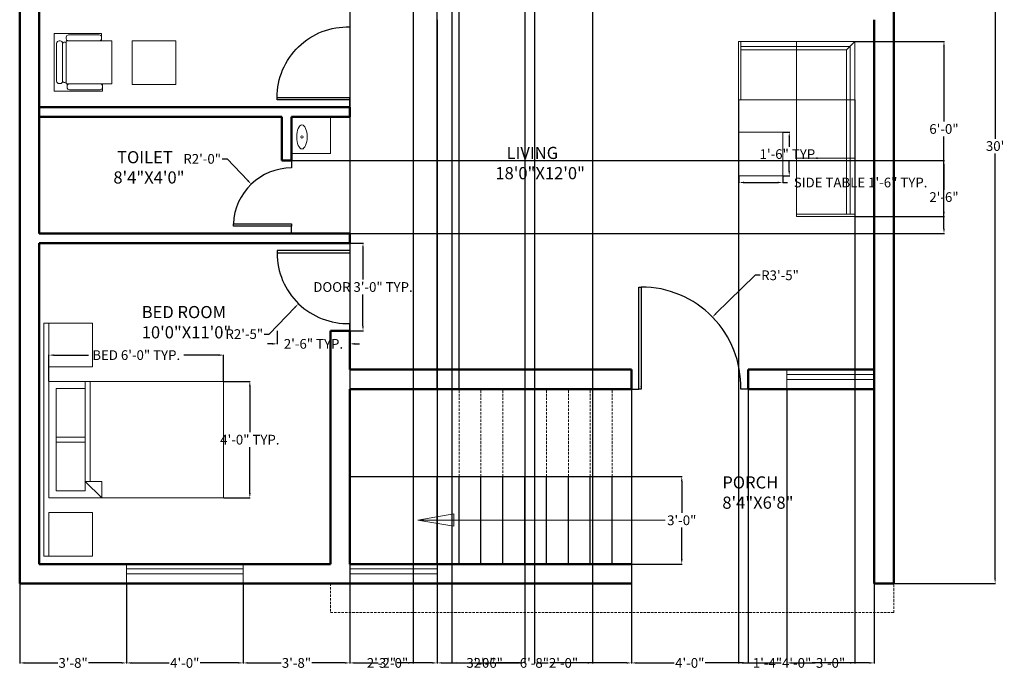
# Model space of a CAD drawing. Units: inches. Extents: x 284 to 690, y 63 to 494.
# Tile 1 of 2: x 284 to 690, y 63 to 331. Entities that reach past the tile are written whole.
import ezdxf

# ---------------------------------------------------------------- set-up
doc = ezdxf.new("R2010")
doc.units = ezdxf.units.IN
doc.header["$MEASUREMENT"] = 0
doc.linetypes.add('DASHEDX2', pattern=[1.5, 1, -0.5])
for name, color, linetype, lineweight in [('A-ANNO-DIMS', 2, 'Continuous', 18), ('A-ANNO-SYMB', 7, 'Continuous', 18), ('A-AREA-IDEN', 7, 'Continuous', 25), ('A-DOOR', 4, 'Continuous', 25), ('A-FLOR-FIXT', 9, 'Continuous', 18), ('A-FLOR-STRS', 7, 'Continuous', 25), ('A-FLOR-STRS-OVHD', 8, 'DASHEDX2', 18), ('A-FURN', 8, 'Continuous', 18), ('A-GLAZ', 3, 'Continuous', 18), ('A-ROOF-OVHD', 8, 'DASHEDX2', 18), ('A-WALL', 7, 'Continuous', 50)]:
    doc.layers.add(name, color=color, linetype=linetype, lineweight=lineweight)
doc.styles.get("Standard").update_dxf_attribs({"font": 'arial.ttf'})
doc.dimstyles.get("Standard").update_dxf_attribs({"dimtxt": 4, "dimasz": 2, "dimexe": 0.18, "dimexo": 0.0625, "dimgap": 1, "dimtad": 0, "dimtih": 1, "dimtoh": 1, "dimdec": 0, "dimzin": 0, "dimdsep": 46, "dimlunit": 3, "dimtxsty": 'Standard', "dimcen": 0.09, "dimadec": 0, "dimazin": 0, "dimtfac": 1, "dimtdec": 0, "dimtofl": 0, "dimtmove": 0, "dimatfit": 3, "dimfxl": 1, "dimtolj": 1, "dimtzin": 0, "dimarcsym": 0})

# ---------------------------------------------------------------- blocks, each defined once
blk = doc.blocks.new('*D2')
at = {"layer": 'A-ANNO-DIMS', "color": 0, "lineweight": -2, "transparency": 16777216}
for p, q in [((644.47, 458.55), (686.36, 458.55)), ((686.18, 456.55), (686.18, 281.59)), ((686.18, 100.55), (686.18, 275.51)), ((644.47, 98.55), (686.36, 98.55))]:
    blk.add_line(p, q, dxfattribs=at)
at = {"layer": 'A-ANNO-DIMS', "color": 0, "lineweight": -3, "transparency": 16777216}
for points in [[(685.85, 456.55), (686.51, 456.55), (686.18, 458.55)], [(685.85, 100.55), (686.51, 100.55), (686.18, 98.55)]]:
    blk.add_solid(points, dxfattribs=at)
at = {"layer": 'Defpoints', "color": 0, "lineweight": -3, "transparency": 16777216}
for p in [(644.41, 458.55), (644.41, 98.55), (686.18, 98.55)]:
    blk.add_point(p, dxfattribs=at)
at = {"layer": 'A-ANNO-DIMS', "color": 0, "transparency": 16777216, "insert": (686.18, 278.55), "char_height": 4, "attachment_point": 5}
blk.add_mtext("\\A1;30'", dxfattribs=at)
blk = doc.blocks.new('BED-48X72')
for p, q in [((0, 0), (0, 72)), ((0, 72), (48, 72)), ((23, 69), (23, 57)), ((25, 69), (25, 57)), ((45, 69), (45, 57)), ((48, 72), (48, 0)), ((0, 50.17), (6.83, 57)), ((45, 57), (3, 57)), ((6.83, 57), (6.83, 50.17)), ((45, 57), (48, 57)), ((48, 57), (48, 54)), ((48, 55), (6.83, 55)), ((0, 50.17), (6.83, 50.17)), ((48, 0), (0, 0))]:
    blk.add_line(p, q)
blk.add_lwpolyline([(3, 57), (3, 69), (45, 69), (45, 57)])
blk = doc.blocks.new('DOOR-SINGLE-30')
for p, q in [((30, 33), (0, 33)), ((0, 33), (0, 32)), ((30, 36), (30, 33)), ((30, 33), (30, 32)), ((0, 32), (30, 32)), ((30, 0), (30, 3))]:
    blk.add_line(p, q)
blk.add_arc((29.02, 32), 29.02, 180, 271.942)
blk = doc.blocks.new('TABLE-SIDE-18SQ')
blk.add_lwpolyline([(18, 18), (18, 0), (0, 0), (0, 18)], close=True)
blk = doc.blocks.new('*D7')
at = {"layer": 'A-ANNO-DIMS', "color": 0, "lineweight": -2, "transparency": 16777216}
for p, q in [((580.68, 266.19), (580.68, 263.37)), ((598.68, 266.19), (598.68, 263.37)), ((582.68, 263.55), (596.68, 263.55)), ((598.68, 263.55), (600.68, 263.55))]:
    blk.add_line(p, q, dxfattribs=at)
at = {"layer": 'A-ANNO-DIMS', "color": 0, "lineweight": -3, "transparency": 16777216}
for points in [[(582.68, 263.88), (582.68, 263.22), (580.68, 263.55)], [(596.68, 263.88), (596.68, 263.22), (598.68, 263.55)]]:
    blk.add_solid(points, dxfattribs=at)
at = {"layer": 'Defpoints', "color": 0, "lineweight": -3, "transparency": 16777216}
for p in [(580.68, 266.25), (598.68, 266.25), (598.68, 263.55)]:
    blk.add_point(p, dxfattribs=at)
at = {"layer": 'A-ANNO-DIMS', "color": 0, "transparency": 16777216, "insert": (630.78, 263.55), "char_height": 4, "attachment_point": 5}
blk.add_mtext('\\A1;SIDE TABLE 1\'-6" TYP.', dxfattribs=at)
blk = doc.blocks.new('*D8')
at = {"layer": 'A-ANNO-DIMS', "color": 0, "lineweight": -2, "transparency": 16777216}
for p, q in [((598.74, 284.25), (601.56, 284.25)), ((601.38, 282.25), (601.38, 278.29)), ((601.38, 268.25), (601.38, 272.21)), ((598.74, 266.25), (601.56, 266.25))]:
    blk.add_line(p, q, dxfattribs=at)
at = {"layer": 'A-ANNO-DIMS', "color": 0, "lineweight": -3, "transparency": 16777216}
for points in [[(601.04, 282.25), (601.71, 282.25), (601.38, 284.25)], [(601.04, 268.25), (601.71, 268.25), (601.38, 266.25)]]:
    blk.add_solid(points, dxfattribs=at)
at = {"layer": 'Defpoints', "color": 0, "lineweight": -3, "transparency": 16777216}
for p in [(598.68, 284.25), (601.38, 284.25), (598.68, 266.25)]:
    blk.add_point(p, dxfattribs=at)
at = {"layer": 'A-ANNO-DIMS', "color": 0, "transparency": 16777216, "insert": (601.38, 275.25), "char_height": 4, "attachment_point": 5}
blk.add_mtext('\\A1;1\'-6" TYP.', dxfattribs=at)
blk = doc.blocks.new('*D9')
at = {"layer": 'A-ANNO-DIMS', "color": 0, "lineweight": -2, "transparency": 16777216}
for p, q in [((296.41, 181.78), (296.41, 192.7)), ((298.41, 192.52), (312.78, 192.52)), ((366.41, 192.52), (352.03, 192.52)), ((368.41, 181.78), (368.41, 192.7))]:
    blk.add_line(p, q, dxfattribs=at)
at = {"layer": 'A-ANNO-DIMS', "color": 0, "lineweight": -3, "transparency": 16777216}
for points in [[(298.41, 192.85), (298.41, 192.19), (296.41, 192.52)], [(366.41, 192.85), (366.41, 192.19), (368.41, 192.52)]]:
    blk.add_solid(points, dxfattribs=at)
at = {"layer": 'Defpoints', "color": 0, "lineweight": -3, "transparency": 16777216}
for p in [(296.41, 192.52), (296.41, 181.72), (368.41, 181.72)]:
    blk.add_point(p, dxfattribs=at)
at = {"layer": 'A-ANNO-DIMS', "color": 0, "transparency": 16777216, "insert": (332.41, 192.52), "char_height": 4, "attachment_point": 5}
blk.add_mtext('\\A1;BED 6\'-0" TYP.', dxfattribs=at)
blk = doc.blocks.new('*D10')
at = {"layer": 'A-ANNO-DIMS', "color": 0, "lineweight": -2, "transparency": 16777216}
for p, q in [((368.47, 181.72), (379.39, 181.72)), ((379.21, 179.72), (379.21, 160.76)), ((379.21, 135.72), (379.21, 154.68)), ((368.47, 133.72), (379.39, 133.72))]:
    blk.add_line(p, q, dxfattribs=at)
at = {"layer": 'A-ANNO-DIMS', "color": 0, "lineweight": -3, "transparency": 16777216}
for points in [[(378.87, 179.72), (379.54, 179.72), (379.21, 181.72)], [(378.87, 135.72), (379.54, 135.72), (379.21, 133.72)]]:
    blk.add_solid(points, dxfattribs=at)
at = {"layer": 'Defpoints', "color": 0, "lineweight": -3, "transparency": 16777216}
for p in [(368.41, 181.72), (379.21, 181.72), (368.41, 133.72)]:
    blk.add_point(p, dxfattribs=at)
at = {"layer": 'A-ANNO-DIMS', "color": 0, "transparency": 16777216, "insert": (379.21, 157.72), "char_height": 4, "attachment_point": 5}
blk.add_mtext('\\A1;4\'-0" TYP.', dxfattribs=at)
blk = doc.blocks.new('*D11')
at = {"layer": 'A-ANNO-DIMS', "color": 0, "lineweight": -2, "transparency": 16777216}
for p, q in [((420.47, 238.55), (425.99, 238.55)), ((425.81, 236.55), (425.81, 223.62)), ((425.81, 204.55), (425.81, 217.48)), ((420.47, 202.55), (425.99, 202.55))]:
    blk.add_line(p, q, dxfattribs=at)
at = {"layer": 'A-ANNO-DIMS', "color": 0, "lineweight": -3, "transparency": 16777216}
for points in [[(425.47, 236.55), (426.14, 236.55), (425.81, 238.55)], [(425.47, 204.55), (426.14, 204.55), (425.81, 202.55)]]:
    blk.add_solid(points, dxfattribs=at)
at = {"layer": 'Defpoints', "color": 0, "lineweight": -3, "transparency": 16777216}
for p in [(420.41, 238.55), (425.81, 238.55), (420.41, 202.55)]:
    blk.add_point(p, dxfattribs=at)
at = {"layer": 'A-ANNO-DIMS', "color": 0, "transparency": 16777216, "insert": (425.81, 220.55), "char_height": 4, "attachment_point": 5}
blk.add_mtext('\\A1;DOOR 3\'-0" TYP.', dxfattribs=at)
blk = doc.blocks.new('*D12')
at = {"layer": 'A-ANNO-DIMS', "color": 0, "lineweight": -2, "transparency": 16777216}
for p, q in [((390.41, 202.49), (390.41, 196.97)), ((420.41, 202.49), (420.41, 196.97)), ((388.41, 197.15), (386.41, 197.15)), ((422.41, 197.15), (424.41, 197.15))]:
    blk.add_line(p, q, dxfattribs=at)
at = {"layer": 'A-ANNO-DIMS', "color": 0, "lineweight": -3, "transparency": 16777216}
for points in [[(388.41, 197.48), (388.41, 196.82), (390.41, 197.15)], [(422.41, 197.48), (422.41, 196.82), (420.41, 197.15)]]:
    blk.add_solid(points, dxfattribs=at)
at = {"layer": 'Defpoints', "color": 0, "lineweight": -3, "transparency": 16777216}
for p in [(390.41, 202.55), (420.41, 202.55), (420.41, 197.15)]:
    blk.add_point(p, dxfattribs=at)
at = {"layer": 'A-ANNO-DIMS', "color": 0, "transparency": 16777216, "insert": (405.41, 197.15), "char_height": 4, "attachment_point": 5}
blk.add_mtext('\\A1;2\'-6" TYP.', dxfattribs=at)
blk = doc.blocks.new('*D15')
at = {"layer": 'A-ANNO-DIMS', "color": 0, "lineweight": -2, "transparency": 16777216}
for p, q in [((284.41, 98.49), (284.41, 65.67)), ((328.41, 98.49), (328.41, 65.67)), ((286.41, 65.85), (300.09, 65.85)), ((326.41, 65.85), (312.72, 65.85))]:
    blk.add_line(p, q, dxfattribs=at)
at = {"layer": 'A-ANNO-DIMS', "color": 0, "lineweight": -3, "transparency": 16777216}
for points in [[(286.41, 66.18), (286.41, 65.52), (284.41, 65.85)], [(326.41, 66.18), (326.41, 65.52), (328.41, 65.85)]]:
    blk.add_solid(points, dxfattribs=at)
at = {"layer": 'Defpoints', "color": 0, "lineweight": -3, "transparency": 16777216}
for p in [(284.41, 98.55), (328.41, 98.55), (328.41, 65.85)]:
    blk.add_point(p, dxfattribs=at)
at = {"layer": 'A-ANNO-DIMS', "color": 0, "transparency": 16777216, "insert": (306.41, 65.85), "char_height": 4, "attachment_point": 5}
blk.add_mtext('\\A1;3\'-8"', dxfattribs=at)
blk = doc.blocks.new('*D16')
at = {"layer": 'A-ANNO-DIMS', "color": 0, "lineweight": -2, "transparency": 16777216}
for p, q in [((328.41, 98.49), (328.41, 65.67)), ((376.41, 98.49), (376.41, 65.67)), ((330.41, 65.85), (346.01, 65.85)), ((374.41, 65.85), (358.8, 65.85))]:
    blk.add_line(p, q, dxfattribs=at)
at = {"layer": 'A-ANNO-DIMS', "color": 0, "lineweight": -3, "transparency": 16777216}
for points in [[(330.41, 66.18), (330.41, 65.52), (328.41, 65.85)], [(374.41, 66.18), (374.41, 65.52), (376.41, 65.85)]]:
    blk.add_solid(points, dxfattribs=at)
at = {"layer": 'Defpoints', "color": 0, "lineweight": -3, "transparency": 16777216}
for p in [(328.41, 98.55), (376.41, 98.55), (376.41, 65.85)]:
    blk.add_point(p, dxfattribs=at)
at = {"layer": 'A-ANNO-DIMS', "color": 0, "transparency": 16777216, "insert": (352.41, 65.85), "char_height": 4, "attachment_point": 5}
blk.add_mtext('\\A1;4\'-0"', dxfattribs=at)
blk = doc.blocks.new('*D17')
at = {"layer": 'A-ANNO-DIMS', "color": 0, "lineweight": -2, "transparency": 16777216}
for p, q in [((376.41, 98.49), (376.41, 65.67)), ((420.41, 98.49), (420.41, 65.67)), ((378.41, 65.85), (392.09, 65.85)), ((418.41, 65.85), (404.72, 65.85))]:
    blk.add_line(p, q, dxfattribs=at)
at = {"layer": 'A-ANNO-DIMS', "color": 0, "lineweight": -3, "transparency": 16777216}
for points in [[(378.41, 66.18), (378.41, 65.52), (376.41, 65.85)], [(418.41, 66.18), (418.41, 65.52), (420.41, 65.85)]]:
    blk.add_solid(points, dxfattribs=at)
at = {"layer": 'Defpoints', "color": 0, "lineweight": -3, "transparency": 16777216}
for p in [(376.41, 98.55), (420.41, 98.55), (420.41, 65.85)]:
    blk.add_point(p, dxfattribs=at)
at = {"layer": 'A-ANNO-DIMS', "color": 0, "transparency": 16777216, "insert": (398.41, 65.85), "char_height": 4, "attachment_point": 5}
blk.add_mtext('\\A1;3\'-8"', dxfattribs=at)
blk = doc.blocks.new('*D18')
at = {"layer": 'A-ANNO-DIMS', "color": 0, "lineweight": -2, "transparency": 16777216}
for p, q in [((420.41, 98.49), (420.41, 65.67)), ((456.41, 98.49), (456.41, 65.67)), ((422.41, 65.85), (432.09, 65.85)), ((454.41, 65.85), (444.72, 65.85))]:
    blk.add_line(p, q, dxfattribs=at)
at = {"layer": 'A-ANNO-DIMS', "color": 0, "lineweight": -3, "transparency": 16777216}
for points in [[(422.41, 66.18), (422.41, 65.52), (420.41, 65.85)], [(454.41, 66.18), (454.41, 65.52), (456.41, 65.85)]]:
    blk.add_solid(points, dxfattribs=at)
at = {"layer": 'Defpoints', "color": 0, "lineweight": -3, "transparency": 16777216}
for p in [(420.41, 98.55), (456.41, 98.55), (456.41, 65.85)]:
    blk.add_point(p, dxfattribs=at)
at = {"layer": 'A-ANNO-DIMS', "color": 0, "transparency": 16777216, "insert": (438.41, 65.85), "char_height": 4, "attachment_point": 5}
blk.add_mtext('\\A1;3\'-0"', dxfattribs=at)
blk = doc.blocks.new('*D19')
at = {"layer": 'A-ANNO-DIMS', "color": 0, "lineweight": -2, "transparency": 16777216}
for p, q in [((456.41, 106.49), (456.41, 65.67)), ((536.41, 106.49), (536.41, 65.67)), ((458.41, 65.85), (490.08, 65.85)), ((534.41, 65.85), (502.73, 65.85))]:
    blk.add_line(p, q, dxfattribs=at)
at = {"layer": 'A-ANNO-DIMS', "color": 0, "lineweight": -3, "transparency": 16777216}
for points in [[(458.41, 66.18), (458.41, 65.52), (456.41, 65.85)], [(534.41, 66.18), (534.41, 65.52), (536.41, 65.85)]]:
    blk.add_solid(points, dxfattribs=at)
at = {"layer": 'Defpoints', "color": 0, "lineweight": -3, "transparency": 16777216}
for p in [(456.41, 106.55), (536.41, 106.55), (536.41, 65.85)]:
    blk.add_point(p, dxfattribs=at)
at = {"layer": 'A-ANNO-DIMS', "color": 0, "transparency": 16777216, "insert": (496.41, 65.85), "char_height": 4, "attachment_point": 5}
blk.add_mtext('\\A1;6\'-8"', dxfattribs=at)
blk = doc.blocks.new('*D20')
at = {"layer": 'A-ANNO-DIMS', "color": 0, "lineweight": -2, "transparency": 16777216}
for p, q in [((536.41, 178.49), (536.41, 65.67)), ((584.41, 178.49), (584.41, 65.67)), ((538.41, 65.85), (554.01, 65.85)), ((582.41, 65.85), (566.8, 65.85))]:
    blk.add_line(p, q, dxfattribs=at)
at = {"layer": 'A-ANNO-DIMS', "color": 0, "lineweight": -3, "transparency": 16777216}
for points in [[(538.41, 66.18), (538.41, 65.52), (536.41, 65.85)], [(582.41, 66.18), (582.41, 65.52), (584.41, 65.85)]]:
    blk.add_solid(points, dxfattribs=at)
at = {"layer": 'Defpoints', "color": 0, "lineweight": -3, "transparency": 16777216}
for p in [(536.41, 178.55), (584.41, 178.55), (584.41, 65.85)]:
    blk.add_point(p, dxfattribs=at)
at = {"layer": 'A-ANNO-DIMS', "color": 0, "transparency": 16777216, "insert": (560.41, 65.85), "char_height": 4, "attachment_point": 5}
blk.add_mtext('\\A1;4\'-0"', dxfattribs=at)
blk = doc.blocks.new('*D21')
at = {"layer": 'A-ANNO-DIMS', "color": 0, "lineweight": -2, "transparency": 16777216}
for p, q in [((584.41, 178.49), (584.41, 65.67)), ((600.41, 178.49), (600.41, 65.67)), ((582.41, 65.85), (580.41, 65.85)), ((602.41, 65.85), (604.41, 65.85))]:
    blk.add_line(p, q, dxfattribs=at)
at = {"layer": 'A-ANNO-DIMS', "color": 0, "lineweight": -3, "transparency": 16777216}
for points in [[(582.41, 66.18), (582.41, 65.52), (584.41, 65.85)], [(602.41, 66.18), (602.41, 65.52), (600.41, 65.85)]]:
    blk.add_solid(points, dxfattribs=at)
at = {"layer": 'Defpoints', "color": 0, "lineweight": -3, "transparency": 16777216}
for p in [(584.41, 178.55), (600.41, 178.55), (600.41, 65.85)]:
    blk.add_point(p, dxfattribs=at)
at = {"layer": 'A-ANNO-DIMS', "color": 0, "transparency": 16777216, "insert": (592.41, 65.85), "char_height": 4, "attachment_point": 5}
blk.add_mtext('\\A1;1\'-4"', dxfattribs=at)
blk = doc.blocks.new('*D22')
at = {"layer": 'A-ANNO-DIMS', "color": 0, "lineweight": -2, "transparency": 16777216}
for p, q in [((600.41, 178.49), (600.41, 65.67)), ((636.41, 178.49), (636.41, 65.67)), ((602.41, 65.85), (612.09, 65.85)), ((634.41, 65.85), (624.72, 65.85))]:
    blk.add_line(p, q, dxfattribs=at)
at = {"layer": 'A-ANNO-DIMS', "color": 0, "lineweight": -3, "transparency": 16777216}
for points in [[(602.41, 66.18), (602.41, 65.52), (600.41, 65.85)], [(634.41, 66.18), (634.41, 65.52), (636.41, 65.85)]]:
    blk.add_solid(points, dxfattribs=at)
at = {"layer": 'Defpoints', "color": 0, "lineweight": -3, "transparency": 16777216}
for p in [(600.41, 178.55), (636.41, 178.55), (636.41, 65.85)]:
    blk.add_point(p, dxfattribs=at)
at = {"layer": 'A-ANNO-DIMS', "color": 0, "transparency": 16777216, "insert": (618.41, 65.85), "char_height": 4, "attachment_point": 5}
blk.add_mtext('\\A1;3\'-0"', dxfattribs=at)
blk = doc.blocks.new('*D25')
at = {"layer": 'A-ANNO-DIMS', "color": 0, "lineweight": -2, "transparency": 16777216}
for p, q in [((456.41, 330.49), (456.41, 65.67)), ((492.41, 330.49), (492.41, 65.67)), ((458.41, 65.85), (468.09, 65.85)), ((490.41, 65.85), (480.72, 65.85))]:
    blk.add_line(p, q, dxfattribs=at)
at = {"layer": 'A-ANNO-DIMS', "color": 0, "lineweight": -3, "transparency": 16777216}
for points in [[(458.41, 66.18), (458.41, 65.52), (456.41, 65.85)], [(490.41, 66.18), (490.41, 65.52), (492.41, 65.85)]]:
    blk.add_solid(points, dxfattribs=at)
at = {"layer": 'Defpoints', "color": 0, "lineweight": -3, "transparency": 16777216}
for p in [(456.41, 330.55), (492.41, 330.55), (492.41, 65.85)]:
    blk.add_point(p, dxfattribs=at)
at = {"layer": 'A-ANNO-DIMS', "color": 0, "transparency": 16777216, "insert": (474.41, 65.85), "char_height": 4, "attachment_point": 5}
blk.add_mtext('\\A1;3\'-0"', dxfattribs=at)
blk = doc.blocks.new('*D26')
at = {"layer": 'A-ANNO-DIMS', "color": 0, "lineweight": -2, "transparency": 16777216}
for p, q in [((536.47, 142.55), (557.29, 142.55)), ((557.11, 140.55), (557.11, 127.59)), ((557.11, 108.55), (557.11, 121.51)), ((536.47, 106.55), (557.29, 106.55))]:
    blk.add_line(p, q, dxfattribs=at)
at = {"layer": 'A-ANNO-DIMS', "color": 0, "lineweight": -3, "transparency": 16777216}
for points in [[(556.77, 140.55), (557.44, 140.55), (557.11, 142.55)], [(556.77, 108.55), (557.44, 108.55), (557.11, 106.55)]]:
    blk.add_solid(points, dxfattribs=at)
at = {"layer": 'Defpoints', "color": 0, "lineweight": -3, "transparency": 16777216}
for p in [(536.41, 142.55), (536.41, 106.55), (557.11, 106.55)]:
    blk.add_point(p, dxfattribs=at)
at = {"layer": 'A-ANNO-DIMS', "color": 0, "transparency": 16777216, "insert": (557.11, 124.55), "char_height": 4, "attachment_point": 5}
blk.add_mtext('\\A1;3\'-0"', dxfattribs=at)
blk = doc.blocks.new('*D27')
at = {"layer": 'A-ANNO-DIMS', "color": 0, "lineweight": -2, "transparency": 16777216}
for p, q in [((456.41, 178.61), (456.41, 479.43)), ((458.41, 479.25), (463.41, 479.25)), ((465.41, 178.61), (465.41, 479.43)), ((465.41, 479.25), (467.41, 479.25))]:
    blk.add_line(p, q, dxfattribs=at)
at = {"layer": 'A-ANNO-DIMS', "color": 0, "lineweight": -3, "transparency": 16777216}
for points in [[(458.41, 479.58), (458.41, 478.92), (456.41, 479.25)], [(463.41, 479.58), (463.41, 478.92), (465.41, 479.25)]]:
    blk.add_solid(points, dxfattribs=at)
at = {"layer": 'Defpoints', "color": 0, "lineweight": -3, "transparency": 16777216}
for p in [(465.41, 479.25), (456.41, 178.55), (465.41, 178.55)]:
    blk.add_point(p, dxfattribs=at)
at = {"layer": 'A-ANNO-DIMS', "color": 0, "transparency": 16777216, "insert": (473.72, 479.25), "char_height": 4, "attachment_point": 5}
blk.add_mtext('\\A1;0\'-9"', dxfattribs=at)
blk = doc.blocks.new('*D28')
at = {"layer": 'A-ANNO-DIMS', "color": 0, "lineweight": -2, "transparency": 16777216}
for p, q in [((396.47, 272.55), (665.29, 272.55)), ((665.11, 270.55), (665.11, 260.59)), ((665.11, 244.55), (665.11, 254.51)), ((396.47, 242.55), (665.29, 242.55))]:
    blk.add_line(p, q, dxfattribs=at)
at = {"layer": 'A-ANNO-DIMS', "color": 0, "lineweight": -3, "transparency": 16777216}
for points in [[(664.77, 270.55), (665.44, 270.55), (665.11, 272.55)], [(664.77, 244.55), (665.44, 244.55), (665.11, 242.55)]]:
    blk.add_solid(points, dxfattribs=at)
at = {"layer": 'Defpoints', "color": 0, "lineweight": -3, "transparency": 16777216}
for p in [(396.41, 272.55), (665.11, 272.55), (396.41, 242.55)]:
    blk.add_point(p, dxfattribs=at)
at = {"layer": 'A-ANNO-DIMS', "color": 0, "transparency": 16777216, "insert": (665.11, 257.55), "char_height": 4, "attachment_point": 5}
blk.add_mtext('\\A1;2\'-6"', dxfattribs=at)
blk = doc.blocks.new('*D30')
at = {"layer": 'A-ANNO-DIMS', "color": 0, "lineweight": -2, "transparency": 16777216}
for p, q in [((496.41, 378.49), (496.41, 65.67)), ((520.41, 378.49), (520.41, 65.67)), ((498.41, 65.85), (502.06, 65.85)), ((518.41, 65.85), (514.76, 65.85))]:
    blk.add_line(p, q, dxfattribs=at)
at = {"layer": 'A-ANNO-DIMS', "color": 0, "lineweight": -3, "transparency": 16777216}
for points in [[(498.41, 66.18), (498.41, 65.52), (496.41, 65.85)], [(518.41, 66.18), (518.41, 65.52), (520.41, 65.85)]]:
    blk.add_solid(points, dxfattribs=at)
at = {"layer": 'Defpoints', "color": 0, "lineweight": -3, "transparency": 16777216}
for p in [(496.41, 378.55), (520.41, 378.55), (520.41, 65.85)]:
    blk.add_point(p, dxfattribs=at)
at = {"layer": 'A-ANNO-DIMS', "color": 0, "transparency": 16777216, "insert": (508.41, 65.85), "char_height": 4, "attachment_point": 5}
blk.add_mtext('\\A1;2\'-0"', dxfattribs=at)
blk = doc.blocks.new('*D32')
at = {"layer": 'A-ANNO-DIMS', "color": 0, "lineweight": -2, "transparency": 16777216}
for p, q in [((492.41, 390.49), (492.41, 65.67)), ((462.41, 386.49), (462.41, 65.67)), ((464.41, 65.85), (471.06, 65.85)), ((490.41, 65.85), (483.76, 65.85))]:
    blk.add_line(p, q, dxfattribs=at)
at = {"layer": 'A-ANNO-DIMS', "color": 0, "lineweight": -3, "transparency": 16777216}
for points in [[(464.41, 66.18), (464.41, 65.52), (462.41, 65.85)], [(490.41, 66.18), (490.41, 65.52), (492.41, 65.85)]]:
    blk.add_solid(points, dxfattribs=at)
at = {"layer": 'Defpoints', "color": 0, "lineweight": -3, "transparency": 16777216}
for p in [(492.41, 390.55), (462.41, 386.55), (492.41, 65.85)]:
    blk.add_point(p, dxfattribs=at)
at = {"layer": 'A-ANNO-DIMS', "color": 0, "transparency": 16777216, "insert": (477.41, 65.85), "char_height": 4, "attachment_point": 5}
blk.add_mtext('\\A1;2\'-6"', dxfattribs=at)
blk = doc.blocks.new('*D33')
at = {"layer": 'A-ANNO-DIMS', "color": 0, "lineweight": -2, "transparency": 16777216}
for p, q in [((420.41, 334.49), (420.41, 65.67)), ((446.41, 334.49), (446.41, 65.67)), ((422.41, 65.85), (427.06, 65.85)), ((444.41, 65.85), (439.76, 65.85))]:
    blk.add_line(p, q, dxfattribs=at)
at = {"layer": 'A-ANNO-DIMS', "color": 0, "lineweight": -3, "transparency": 16777216}
for points in [[(422.41, 66.18), (422.41, 65.52), (420.41, 65.85)], [(444.41, 66.18), (444.41, 65.52), (446.41, 65.85)]]:
    blk.add_solid(points, dxfattribs=at)
at = {"layer": 'Defpoints', "color": 0, "lineweight": -3, "transparency": 16777216}
for p in [(420.41, 334.55), (446.41, 334.55), (446.41, 65.85)]:
    blk.add_point(p, dxfattribs=at)
at = {"layer": 'A-ANNO-DIMS', "color": 0, "transparency": 16777216, "insert": (433.41, 65.85), "char_height": 4, "attachment_point": 5}
blk.add_mtext('\\A1;2\'-2"', dxfattribs=at)
blk = doc.blocks.new('*D34')
at = {"layer": 'A-ANNO-DIMS', "color": 0, "lineweight": -2, "transparency": 16777216}
for p, q in [((580.42, 297.53), (580.42, 65.67)), ((628.42, 297.53), (628.42, 65.67)), ((582.42, 65.85), (598.02, 65.85)), ((626.42, 65.85), (610.82, 65.85))]:
    blk.add_line(p, q, dxfattribs=at)
at = {"layer": 'A-ANNO-DIMS', "color": 0, "lineweight": -3, "transparency": 16777216}
for points in [[(582.42, 66.18), (582.42, 65.52), (580.42, 65.85)], [(626.42, 66.18), (626.42, 65.52), (628.42, 65.85)]]:
    blk.add_solid(points, dxfattribs=at)
at = {"layer": 'Defpoints', "color": 0, "lineweight": -3, "transparency": 16777216}
for p in [(580.42, 297.59), (628.42, 297.59), (628.42, 65.85)]:
    blk.add_point(p, dxfattribs=at)
at = {"layer": 'A-ANNO-DIMS', "color": 0, "transparency": 16777216, "insert": (604.42, 65.85), "char_height": 4, "attachment_point": 5}
blk.add_mtext('\\A1;4\'-0"', dxfattribs=at)
blk = doc.blocks.new('*D35')
at = {"layer": 'A-ANNO-DIMS', "color": 0, "lineweight": -2, "transparency": 16777216}
for p, q in [((628.48, 321.59), (665.29, 321.59)), ((665.11, 319.59), (665.11, 288.63)), ((665.11, 251.59), (665.11, 282.55)), ((628.48, 249.59), (665.29, 249.59))]:
    blk.add_line(p, q, dxfattribs=at)
at = {"layer": 'A-ANNO-DIMS', "color": 0, "lineweight": -3, "transparency": 16777216}
for points in [[(664.77, 319.59), (665.44, 319.59), (665.11, 321.59)], [(664.77, 251.59), (665.44, 251.59), (665.11, 249.59)]]:
    blk.add_solid(points, dxfattribs=at)
at = {"layer": 'Defpoints', "color": 0, "lineweight": -3, "transparency": 16777216}
for p in [(628.42, 321.59), (628.42, 249.59), (665.11, 249.59)]:
    blk.add_point(p, dxfattribs=at)
at = {"layer": 'A-ANNO-DIMS', "color": 0, "transparency": 16777216, "insert": (665.11, 285.59), "char_height": 4, "attachment_point": 5}
blk.add_mtext('\\A1;6\'-0"', dxfattribs=at)
blk = doc.blocks.new('*D36')
at = {"layer": 'A-ANNO-DIMS', "color": 0, "lineweight": -2, "transparency": 16777216}
for p, q in [((587.36, 225.37), (571.18, 209.58)), ((589.36, 225.37), (587.36, 225.37)), ((540.32, 179.54), (540.5, 179.54)), ((540.41, 179.45), (540.41, 179.63))]:
    blk.add_line(p, q, dxfattribs=at)
at = {"layer": 'A-ANNO-DIMS', "color": 0, "lineweight": -3, "transparency": 16777216}
blk.add_solid([(570.95, 209.82), (571.42, 209.34), (569.75, 208.19)], dxfattribs=at)
at = {"layer": 'Defpoints', "color": 0, "lineweight": -3, "transparency": 16777216}
for p in [(569.75, 208.19), (540.41, 179.54)]:
    blk.add_point(p, dxfattribs=at)
at = {"layer": 'A-ANNO-DIMS', "color": 0, "transparency": 16777216, "insert": (597.59, 225.37), "char_height": 4, "attachment_point": 5}
blk.add_mtext('\\A1;R3\'-5"', dxfattribs=at)
blk = doc.blocks.new('*D37')
at = {"layer": 'A-ANNO-DIMS', "color": 0, "lineweight": -2, "transparency": 16777216}
for p, q in [((419.33, 234.55), (419.51, 234.55)), ((419.42, 234.46), (419.42, 234.64)), ((387.15, 201.17), (397.86, 212.25)), ((385.15, 201.17), (387.15, 201.17))]:
    blk.add_line(p, q, dxfattribs=at)
at = {"layer": 'A-ANNO-DIMS', "color": 0, "lineweight": -3, "transparency": 16777216}
blk.add_solid([(397.63, 212.48), (398.1, 212.02), (399.26, 213.69)], dxfattribs=at)
at = {"layer": 'Defpoints', "color": 0, "lineweight": -3, "transparency": 16777216}
for p in [(419.42, 234.55), (399.26, 213.69)]:
    blk.add_point(p, dxfattribs=at)
at = {"layer": 'A-ANNO-DIMS', "color": 0, "transparency": 16777216, "insert": (376.92, 201.17), "char_height": 4, "attachment_point": 5}
blk.add_mtext('\\A1;R2\'-5"', dxfattribs=at)
blk = doc.blocks.new('*D38')
at = {"layer": 'A-ANNO-DIMS', "color": 0, "lineweight": -2, "transparency": 16777216}
for p, q in [((367.81, 273.28), (369.81, 273.28)), ((369.81, 273.28), (378.4, 264.32)), ((396.32, 245.53), (396.5, 245.53)), ((396.41, 245.44), (396.41, 245.62))]:
    blk.add_line(p, q, dxfattribs=at)
at = {"layer": 'A-ANNO-DIMS', "color": 0, "lineweight": -3, "transparency": 16777216}
blk.add_solid([(378.64, 264.55), (378.16, 264.08), (379.78, 262.87)], dxfattribs=at)
at = {"layer": 'Defpoints', "color": 0, "lineweight": -3, "transparency": 16777216}
for p in [(379.78, 262.87), (396.41, 245.53)]:
    blk.add_point(p, dxfattribs=at)
at = {"layer": 'A-ANNO-DIMS', "color": 0, "transparency": 16777216, "insert": (359.58, 273.28), "char_height": 4, "attachment_point": 5}
blk.add_mtext('\\A1;R2\'-0"', dxfattribs=at)

msp = doc.modelspace()

# ---------------------------------------------------------------- linework, layer by layer
at = {"layer": 'A-ANNO-SYMB'}
for p, q in [((448.41, 124.55), (463.18, 127.17)), ((463.18, 127.17), (463.2, 122.06)), ((456.41, 124.55), (448.41, 124.55)), ((448.41, 124.55), (463.2, 122.06)), ((456.41, 124.55), (550.22, 124.55))]:
    msp.add_line(p, q, dxfattribs=at)
at = {"layer": 'A-DOOR'}
for p, q in [((396.41, 272.55), (396.41, 269.55)), ((372.41, 245.55), (372.41, 246.55)), ((372.41, 246.55), (396.41, 246.55)), ((396.41, 245.55), (372.41, 245.55)), ((396.41, 246.55), (396.41, 245.55)), ((396.41, 242.55), (396.41, 245.55)), ((539.41, 178.55), (539.41, 220.55)), ((539.41, 220.55), (540.41, 220.55)), ((540.41, 220.55), (540.41, 178.55)), ((536.41, 178.55), (539.41, 178.55)), ((540.41, 178.55), (539.41, 178.55)), ((584.41, 178.55), (581.41, 178.55))]:
    msp.add_line(p, q, dxfattribs=at)
for centre, radius, start, end in [((396.41, 245.53), 24.02, 90, 177.5622), ((540.41, 179.54), 41.01, 358.6194, 90)]:
    msp.add_arc(centre, radius, start, end, dxfattribs=at)
at = {"layer": 'A-FLOR-FIXT'}
for p, q in [((412.41, 275.55), (412.41, 290.55)), ((396.41, 275.55), (412.41, 275.55))]:
    msp.add_line(p, q, dxfattribs=at)
msp.add_circle((400.67, 282.31), 0.5, dxfattribs=at)
msp.add_ellipse((400.67, 282.31), major_axis=(0, 4.94), ratio=0.435239, dxfattribs=at)
at = {"layer": 'A-FLOR-STRS'}
for p, q in [((420.41, 142.55), (536.41, 142.55)), ((456.41, 106.55), (456.41, 142.55)), ((465.41, 106.55), (465.41, 142.55)), ((474.41, 106.55), (474.41, 142.55)), ((483.41, 106.55), (483.41, 142.55)), ((492.41, 106.55), (492.41, 142.55)), ((501.41, 106.55), (501.41, 142.55)), ((510.41, 106.55), (510.41, 142.55)), ((510.41, 106.55), (510.41, 142.55)), ((510.41, 106.55), (510.41, 142.55)), ((519.41, 106.55), (519.41, 142.55)), ((528.41, 106.55), (528.41, 142.55)), ((536.41, 142.55), (536.41, 98.55)), ((420.41, 106.55), (456.41, 106.55))]:
    msp.add_line(p, q, dxfattribs=at)
at = {"layer": 'A-FLOR-STRS-OVHD'}
for p, q in [((456.41, 142.55), (456.41, 178.55)), ((465.41, 142.55), (465.41, 178.55)), ((474.41, 142.55), (474.41, 178.55)), ((483.41, 142.55), (483.41, 178.55)), ((492.41, 142.55), (492.41, 178.55)), ((501.41, 142.55), (501.41, 178.55)), ((510.41, 142.55), (510.41, 178.55)), ((519.41, 142.55), (519.41, 178.55)), ((528.41, 142.55), (528.41, 178.55)), ((536.41, 142.55), (536.41, 178.55))]:
    msp.add_line(p, q, dxfattribs=at)
at = {"layer": 'A-FURN'}
for p, q in [((299.63, 324.86), (298.63, 324.86)), ((298.63, 324.86), (298.63, 304.18)), ((318.14, 324.86), (299.63, 324.86)), ((318.14, 321.86), (318.14, 324.86)), ((299.63, 305.23), (299.63, 320.81)), ((300.63, 321.81), (301.1, 321.81)), ((302.1, 320.81), (302.1, 305.23)), ((302.1, 305.23), (302.1, 320.81)), ((302.6, 321.31), (303.06, 321.31)), ((303.56, 323.33), (303.56, 322.86)), ((303.56, 321.86), (310.85, 321.86)), ((303.56, 304.18), (303.56, 321.86)), ((303.56, 320.81), (303.56, 305.23)), ((310.85, 324.33), (304.56, 324.33)), ((304.56, 321.86), (310.85, 321.86)), ((317.14, 324.33), (310.85, 324.33)), ((310.85, 321.86), (317.14, 321.86)), ((310.85, 321.86), (322.39, 321.86)), ((318.14, 322.86), (318.14, 323.33)), ((322.39, 321.86), (322.39, 304.18)), ((604.42, 321.59), (580.42, 321.59)), ((580.42, 321.59), (580.42, 297.59)), ((581.42, 321.59), (581.42, 297.59)), ((628.42, 321.59), (604.42, 321.59)), ((604.42, 321.59), (604.42, 249.59)), ((624.92, 318.09), (628.42, 321.59)), ((628.42, 249.59), (628.42, 321.59)), ((604.42, 319.59), (581.42, 319.59)), ((604.42, 318.09), (581.42, 318.09)), ((626.42, 319.59), (604.42, 319.59)), ((624.92, 318.09), (604.42, 318.09)), ((624.92, 250.59), (624.92, 318.09)), ((626.42, 250.59), (626.42, 319.59)), ((298.63, 304.18), (298.63, 301.18)), ((301.1, 304.23), (300.63, 304.23)), ((303.06, 304.73), (302.6, 304.73)), ((310.85, 304.18), (303.56, 304.18)), ((310.85, 304.18), (304.93, 304.18)), ((322.39, 304.18), (310.85, 304.18)), ((317.5, 304.18), (310.85, 304.18)), ((310.85, 304.18), (310.85, 304.18)), ((310.85, 304.18), (310.85, 304.18)), ((318.5, 301.18), (318.5, 304.18)), ((298.63, 301.18), (318.5, 301.18)), ((303.93, 303.18), (303.93, 302.72)), ((304.93, 301.72), (310.85, 301.72)), ((310.85, 301.72), (317.5, 301.72)), ((318.5, 302.72), (318.5, 303.18)), ((580.42, 297.59), (604.42, 297.59)), ((604.42, 297.59), (628.42, 297.59)), ((604.42, 273.59), (628.42, 273.59)), ((604.42, 250.59), (628.42, 250.59)), ((604.42, 249.59), (628.42, 249.59)), ((294.41, 109.72), (294.41, 205.72)), ((296.41, 205.72), (294.41, 205.72)), ((296.41, 109.72), (294.41, 109.72))]:
    msp.add_line(p, q, dxfattribs=at)
for centre, radius, start, end in [((300.63, 320.81), 1, 90, 180), ((301.1, 320.81), 1, 0, 90), ((302.6, 320.81), 0.5, 90, 180), ((303.06, 320.81), 0.5, 0, 90), ((304.56, 323.33), 1, 90, 180), ((304.56, 322.86), 1, 180, 270), ((317.14, 323.33), 1, 0, 90), ((317.14, 322.86), 1, 270, 0), ((300.63, 305.23), 1, 180, 270), ((301.1, 305.23), 1, 270, 0), ((302.6, 305.23), 0.5, 180, 270), ((303.06, 305.23), 0.5, 270, 0), ((304.93, 303.18), 1, 90, 180), ((317.5, 303.18), 1, 0, 90), ((304.93, 302.72), 1, 180, 270), ((317.5, 302.72), 1, 270, 0)]:
    msp.add_arc(centre, radius, start, end, dxfattribs=at)
at = {"layer": 'A-GLAZ'}
for p, q in [((600.41, 178.55), (600.41, 186.55)), ((600.41, 184.55), (636.41, 184.55)), ((600.41, 182.55), (636.41, 182.55)), ((328.41, 106.55), (328.41, 98.55)), ((376.41, 106.55), (376.41, 98.55)), ((420.41, 106.55), (420.41, 98.55)), ((456.41, 106.55), (456.41, 98.55)), ((328.41, 104.55), (376.41, 104.55)), ((328.41, 102.55), (376.41, 102.55)), ((420.41, 104.55), (456.41, 104.55)), ((420.41, 102.55), (456.41, 102.55))]:
    msp.add_line(p, q, dxfattribs=at)
at = {"layer": 'A-ROOF-OVHD'}
for p, q in [((412.41, 98.55), (412.41, 86.55)), ((644.41, 86.55), (644.41, 98.55)), ((412.41, 86.55), (644.41, 86.55))]:
    msp.add_line(p, q, dxfattribs=at)
at = {"layer": 'A-WALL'}
for p, q in [((284.41, 98.55), (284.41, 458.55)), ((644.41, 458.55), (644.41, 98.55)), ((292.41, 242.55), (292.41, 450.55)), ((636.41, 98.55), (636.41, 330.55)), ((420.41, 294.55), (292.41, 294.55)), ((420.41, 290.55), (420.41, 294.55)), ((392.41, 290.55), (292.41, 290.55)), ((392.41, 290.55), (392.41, 272.55)), ((420.41, 290.55), (396.41, 290.55)), ((396.41, 290.55), (396.41, 272.55)), ((392.41, 272.55), (396.41, 272.55)), ((420.41, 242.55), (292.41, 242.55)), ((420.41, 242.55), (420.41, 238.55)), ((292.41, 106.55), (292.41, 238.55)), ((420.41, 238.55), (292.41, 238.55)), ((412.41, 106.55), (412.41, 202.55)), ((412.41, 202.55), (420.41, 202.55)), ((420.41, 186.55), (420.41, 202.55)), ((536.41, 186.55), (420.41, 186.55)), ((536.41, 178.55), (536.41, 186.55)), ((636.41, 186.55), (584.41, 186.55)), ((584.41, 178.55), (584.41, 186.55)), ((420.41, 106.55), (420.41, 178.55)), ((536.41, 178.55), (420.41, 178.55)), ((636.41, 178.55), (584.41, 178.55)), ((412.41, 106.55), (292.41, 106.55)), ((536.41, 106.55), (420.41, 106.55)), ((536.41, 98.55), (284.41, 98.55)), ((644.41, 98.55), (636.41, 98.55))]:
    msp.add_line(p, q, dxfattribs=at)

# ---------------------------------------------------------------- block references
at = {"layer": 'A-DOOR', "extrusion": (0, 0, -1), "zscale": -1, "rotation": 180}
msp.add_blockref('DOOR-SINGLE-30', (-390.41, 330.55), dxfattribs=at)
at = {"layer": 'A-DOOR'}
msp.add_blockref('DOOR-SINGLE-30', (390.41, 202.55), dxfattribs=at)
at = {"layer": 'A-FURN'}
for name, p, rotation in [('TABLE-SIDE-18SQ', (348.77, 303.86), 90), ('TABLE-SIDE-18SQ', (314.41, 187.72), 90.00000000000017), ('BED-48X72', (368.41, 133.72), 90.0000000000003), ('TABLE-SIDE-18SQ', (314.41, 109.72), 90.00000000000017)]:
    msp.add_blockref(name, p, dxfattribs=dict(at, rotation=rotation))
msp.add_blockref('TABLE-SIDE-18SQ', (580.68, 266.25), dxfattribs=at)

# ---------------------------------------------------------------- texts
at = {"layer": 'A-AREA-IDEN', "char_height": 5, "attachment_point": 1}
for s, insert in [(' TOILET\\P8\'4"X4\'0"', (322.99, 276.47)), ('   LIVING\\P18\'0"X12\'0"', (480.34, 278.23)), ('BED ROOM\\P10\'0"X11\'0"', (334.68, 212.73)), ('PORCH\\P8\'4"X6\'8"', (573.82, 142.63))]:
    msp.add_mtext_dynamic_manual_height_columns(s, width=85.9248, gutter_width=1, heights=[0], dxfattribs=dict(at, insert=insert))

# ---------------------------------------------------------------- dimensions: what is measured, and where the dimension line sits
at = {"layer": 'A-ANNO-DIMS'}
for base, p1, p2, picture, middle in [((465.41, 479.25), (456.41, 178.55), (465.41, 178.55), '*D27', (473.72, 479.25)), ((492.41, 65.85), (462.41, 386.55), (492.41, 390.55), '*D32', (477.41, 65.85)), ((520.41, 65.85), (496.41, 378.55), (520.41, 378.55), '*D30', (508.41, 65.85)), ((446.41, 65.85), (420.41, 334.55), (446.41, 334.55), '*D33', (433.41, 65.85)), ((492.41, 65.85), (456.41, 330.55), (492.41, 330.55), '*D25', (474.41, 65.85)), ((628.42, 65.85), (580.42, 297.59), (628.42, 297.59), '*D34', (604.42, 65.85)), ((584.41, 65.85), (536.41, 178.55), (584.41, 178.55), '*D20', (560.41, 65.85)), ((600.41, 65.85), (584.41, 178.55), (600.41, 178.55), '*D21', (592.41, 65.85)), ((636.41, 65.85), (600.41, 178.55), (636.41, 178.55), '*D22', (618.41, 65.85)), ((536.41, 65.85), (456.41, 106.55), (536.41, 106.55), '*D19', (496.41, 65.85)), ((328.41, 65.85), (284.41, 98.55), (328.41, 98.55), '*D15', (306.41, 65.85)), ((376.41, 65.85), (328.41, 98.55), (376.41, 98.55), '*D16', (352.41, 65.85)), ((420.41, 65.85), (376.41, 98.55), (420.41, 98.55), '*D17', (398.41, 65.85)), ((456.41, 65.85), (420.41, 98.55), (456.41, 98.55), '*D18', (438.41, 65.85))]:
    dim = msp.add_linear_dim(base=base, p1=p1, p2=p2, dimstyle='Standard', override={"dimdec": 1, "dimlfac": 1, "dimrnd": 0, "dimzin": 1, "dimdsep": 46, "dimlunit": 4, "dimfrac": 2}, dxfattribs=at)
    dim.commit()
    dim.dimension.update_dxf_attribs({"geometry": picture, "text_midpoint": middle})
for base, p1, p2, angle, override, picture, middle in [((686.18, 98.55), (644.41, 458.55), (644.41, 98.55), 90, {"dimclrd": 0, "dimclre": 0, "dimclrt": 0}, '*D2', (686.18, 278.55)), ((665.11, 249.59), (628.42, 321.59), (628.42, 249.59), 90, {"dimdec": 1, "dimlfac": 1, "dimrnd": 0, "dimzin": 1, "dimdsep": 46, "dimlunit": 4, "dimfrac": 2}, '*D35', (665.11, 285.59)), ((665.11, 272.55), (396.41, 242.55), (396.41, 272.55), 90, {"dimdec": 1, "dimlfac": 1, "dimrnd": 0, "dimzin": 1, "dimdsep": 46, "dimlunit": 4, "dimfrac": 2}, '*D28', (665.11, 257.55)), ((557.11, 106.55), (536.41, 142.55), (536.41, 106.55), 270, {"dimdec": 1, "dimlfac": 1, "dimrnd": 0, "dimzin": 1, "dimdsep": 46, "dimlunit": 4, "dimfrac": 2}, '*D26', (557.11, 124.55))]:
    dim = msp.add_linear_dim(base=base, p1=p1, p2=p2, angle=angle, dimstyle='Standard', override=override, dxfattribs=at)
    dim.commit()
    dim.dimension.update_dxf_attribs({"geometry": picture, "text_midpoint": middle})
for base, p1, p2, angle, text, picture, middle in [((601.38, 284.25), (598.68, 266.25), (598.68, 284.25), 90, '<> TYP.', '*D8', (601.38, 275.25)), ((425.81, 238.55), (420.41, 202.55), (420.41, 238.55), 90, 'DOOR <> TYP.', '*D11', (425.81, 220.55)), ((296.41, 192.52), (368.41, 181.72), (296.41, 181.72), 180, 'BED <> TYP.', '*D9', (332.41, 192.52)), ((379.21, 181.72), (368.41, 133.72), (368.41, 181.72), 90, '<> TYP.', '*D10', (379.21, 157.72))]:
    dim = msp.add_linear_dim(base=base, p1=p1, p2=p2, angle=angle, text=text, dimstyle='Standard', override={"dimdec": 1, "dimlfac": 1, "dimrnd": 0, "dimzin": 1, "dimdsep": 46, "dimlunit": 4, "dimfrac": 2}, dxfattribs=at)
    dim.commit()
    dim.dimension.update_dxf_attribs({"geometry": picture, "text_midpoint": middle})
for center, mpoint, picture, middle in [((396.41, 245.53), (379.78, 262.87), '*D38', (359.58, 273.28)), ((419.42, 234.55), (399.26, 213.69), '*D37', (376.92, 201.17)), ((540.41, 179.54), (569.75, 208.19), '*D36', (597.59, 225.37))]:
    dim = msp.add_radius_dim(center=center, mpoint=mpoint, dimstyle='Standard', override={"dimdec": 1, "dimlfac": 1, "dimrnd": 0, "dimzin": 1, "dimdsep": 46, "dimlunit": 4, "dimfrac": 2}, dxfattribs=at)
    dim.commit()
    dim.dimension.update_dxf_attribs({"geometry": picture, "text_midpoint": middle, "dimtype": 164})
for base, p1, p2, text, picture, middle in [((598.68, 263.55), (580.68, 266.25), (598.68, 266.25), 'SIDE TABLE <> TYP.', '*D7', (630.78, 263.55)), ((420.41, 197.15), (390.41, 202.55), (420.41, 202.55), '<> TYP.', '*D12', (405.41, 197.15))]:
    dim = msp.add_linear_dim(base=base, p1=p1, p2=p2, text=text, dimstyle='Standard', override={"dimdec": 1, "dimlfac": 1, "dimrnd": 0, "dimzin": 1, "dimdsep": 46, "dimlunit": 4, "dimfrac": 2}, dxfattribs=at)
    dim.commit()
    dim.dimension.update_dxf_attribs({"geometry": picture, "text_midpoint": middle})

doc.saveas('drawing.dxf')
